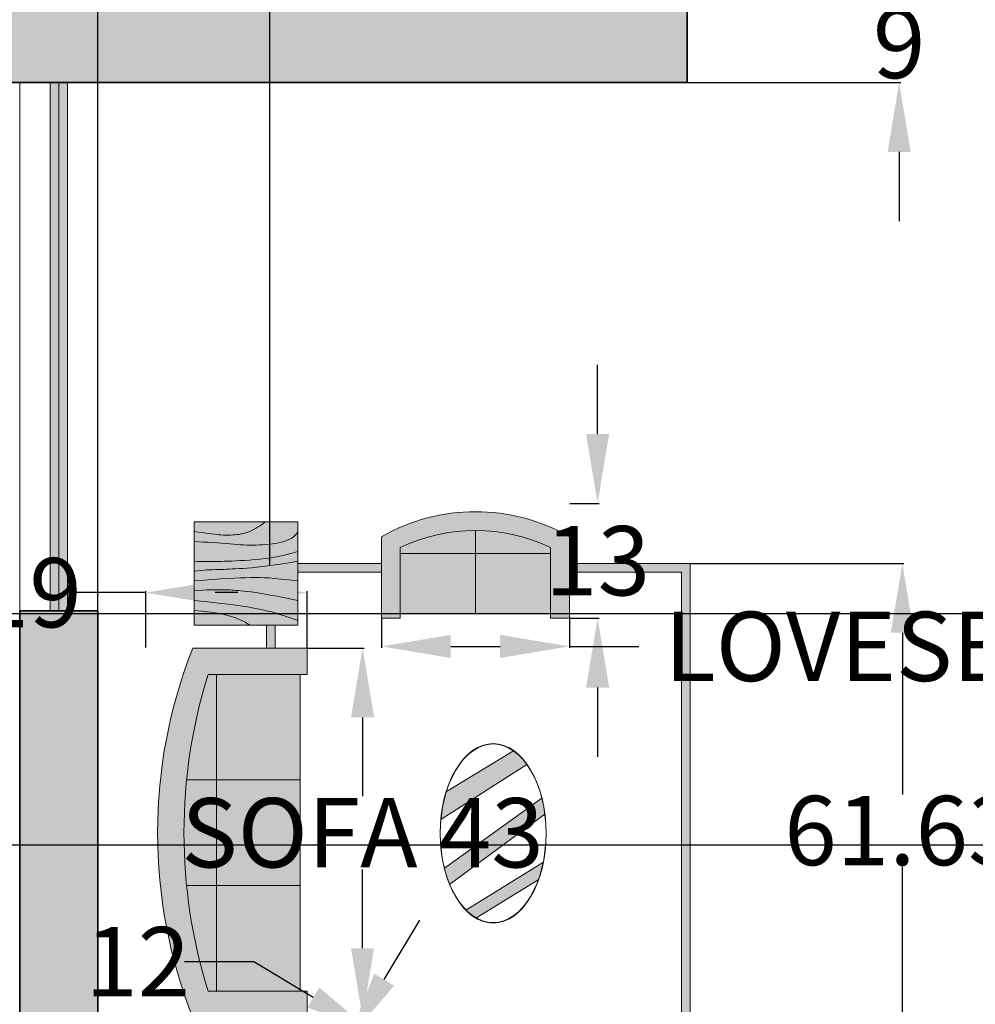
# Model space of a CAD drawing. Units: inches. Extents: x -52 to 678, y 23 to 685.
# Tile 4 of 11: x 189 to 299, y 221 to 334. Entities that reach past the tile are written whole.
import ezdxf

# ---------------------------------------------------------------- set-up
doc = ezdxf.new("R2010")
doc.units = ezdxf.units.IN
doc.header["$MEASUREMENT"] = 0
for name, color, linetype, lineweight in [('A-ANNO-DIMS', 2, 'Continuous', 18), ('A-FURN', 8, 'Continuous', 18), ('A-FURN-PATT', 252, 'Continuous', 13), ('A-GLAZ', 4, 'Continuous', 18), ('A-WALL', 7, 'Continuous', 35)]:
    doc.layers.add(name, color=color, linetype=linetype, lineweight=lineweight)
doc.layers.add('A-GLAZ-PATT', color=18, linetype='Continuous', lineweight=13, true_color=0x000000)
doc.layers.add('A-WALL-PATT', color=18, linetype='Continuous', lineweight=13, true_color=0x000000)
doc.styles.get("Standard").update_dxf_attribs({"font": 'arial.ttf'})
doc.dimstyles.get("Standard").update_dxf_attribs({"dimtxt": 8, "dimasz": 8, "dimexe": 0.18, "dimexo": 0.0625, "dimgap": 0.09, "dimtad": 0, "dimtih": 1, "dimtoh": 1, "dimdec": 0, "dimzin": 0, "dimdsep": 46, "dimlunit": 3, "dimtxsty": 'Standard', "dimcen": 0.09, "dimadec": 0, "dimazin": 0, "dimtfac": 1, "dimtdec": 0, "dimtofl": 0, "dimtmove": 0, "dimatfit": 3, "dimfxl": 1, "dimtolj": 1, "dimtzin": 0, "dimarcsym": 0})

# ---------------------------------------------------------------- blocks, each defined once
blk = doc.blocks.new('Sofa - Roundback Loveseat 5 ft.')
for p, q in [((0, -32.44198), (0, -5.99998)), ((-24, -33.99998), (-24, -11.46958)), ((24.00004, -33.99998), (24.00004, -11.46958)), ((-23.9998, -13.38178), (23.99986, -13.38178)), ((-24, -32.44198), (24.00004, -32.44198))]:
    blk.add_line(p, q)
for points in [[(-24, -33.99998), (-30, -33.99998), (-30, -7.99998)], [(30.00004, -7.99998), (30.00004, -33.99998), (24.00004, -33.99998)]]:
    blk.add_lwpolyline(points)
for centre, radius, start, end in [((0, -60.24998), 60.24998, 60.13715, 119.8628), ((0, -61.38438), 55.38444, 64.32083, 115.6792)]:
    blk.add_arc(centre, radius, start, end)
blk = doc.blocks.new('Sofa - Roundback 7 ft.')
for p, q in [((-12.00002, -32.4421), (-12.00003, -6.5971)), ((11.99997, -32.4421), (11.99998, -6.5971)), ((-36.000027, -34), (-36.000027, -11.4696)), ((-35.999844, -13.3819), (35.9998, -13.3819)), ((35.99998, -34), (35.99998, -11.4696)), ((-36.000027, -32.4421), (35.99998, -32.4421))]:
    blk.add_line(p, q)
for points in [[(-36.000027, -34), (-42.000027, -34), (-42.000027, -8)], [(41.99998, -8), (41.99998, -34), (35.99998, -34)]]:
    blk.add_lwpolyline(points)
for centre, radius, start, end in [((0, -114.25), 114.25, 68.43141, 111.5686), ((-0.00001, -127.1968), 121.1968, 72.72033, 107.2797)]:
    blk.add_arc(centre, radius, start, end)
blk = doc.blocks.new('Table - Square Woodgrain 42 x 42 in.')
blk.add_line((0, -42), (42, -42))
for points in [[(0, -4), (1.704, -4.2172), (3.2358, -4.4188), (4.615, -4.604), (5.8615, -4.7721), (6.9951, -4.9224), (8.0357, -5.0541), (9.0031, -5.1667), (9.9171, -5.2594), (10.7951, -5.3316), (11.6445, -5.3836), (12.4702, -5.4157), (13.277, -5.4283), (14.0698, -5.4217), (14.8535, -5.3964), (15.6331, -5.3526), (16.4133, -5.2908), (17.1986, -5.2103), (17.9913, -5.1062), (18.793, -4.9727), (19.6056, -4.8038), (20.4307, -4.5937), (21.2701, -4.3365), (22.1256, -4.0262), (22.9989, -3.6571), (23.888, -3.2272), (24.7756, -2.7516), (25.6408, -2.2491), (26.4624, -1.7387), (27.2195, -1.2395), (27.891, -0.7703), (28.456, -0.3501), (28.8934, 0.002)], [(0, -42), (0, 0), (42, 0), (42, -42)], [(0, -8), (1.8203, -8.1001), (3.6741, -8.2149), (5.5411, -8.3408), (7.4011, -8.4741), (9.2339, -8.6112), (11.0193, -8.7484), (12.7371, -8.8821), (14.3671, -9.0086), (15.8954, -9.1246), (17.3337, -9.2278), (18.6997, -9.3159), (20.0116, -9.387), (21.2871, -9.4389), (22.5442, -9.4696), (23.8008, -9.477), (25.0749, -9.459), (26.3791, -9.4137), (27.7049, -9.3403), (29.0383, -9.2382), (30.3655, -9.1068), (31.6728, -8.9455), (32.9461, -8.7535), (34.1717, -8.5304), (35.3358, -8.2756), (36.4268, -7.9863), (37.443, -7.6521), (38.3849, -7.2603), (39.253, -6.7986), (40.048, -6.2542), (40.7705, -5.6147), (41.421, -4.8674), (42, -4)], [(42, -12), (39.1784, -12.8621), (36.4519, -13.5654), (33.8246, -14.1294), (31.3004, -14.5731), (28.8832, -14.9161), (26.577, -15.1775), (24.3858, -15.3768), (22.3136, -15.5332), (20.3622, -15.6632), (18.5254, -15.7718), (16.7947, -15.8612), (15.1618, -15.9338), (13.6183, -15.9916), (12.1558, -16.0369), (10.7659, -16.0718), (9.4403, -16.0987), (8.1703, -16.1191), (6.9461, -16.1325), (5.7577, -16.1377), (4.595, -16.1335), (3.4479, -16.1188), (2.3064, -16.0924), (1.1604, -16.0532), (0, -16)], [(42, -16), (37.6529, -16.7365), (33.8802, -17.329), (30.6179, -17.7961), (27.8015, -18.1561), (25.3668, -18.4275), (23.2497, -18.6288), (21.3859, -18.7785), (19.7111, -18.8949), (18.1693, -18.9939), (16.7375, -19.0795), (15.401, -19.1534), (14.1449, -19.217), (12.9544, -19.2717), (11.8148, -19.3191), (10.7113, -19.3606), (9.6291, -19.3976), (8.5534, -19.4323), (7.47, -19.4689), (6.3643, -19.5122), (5.222, -19.5672), (4.0288, -19.6386), (2.7703, -19.7313), (1.4321, -19.8501), (0, -20)], [(0, -24), (3.9243, -23.6805), (7.4766, -23.4138), (10.6891, -23.1954), (13.5943, -23.0205), (16.2247, -22.8847), (18.6125, -22.7832), (20.7903, -22.7116), (22.7903, -22.6651), (24.6563, -22.642), (26.4764, -22.6507), (28.35, -22.7024), (30.3766, -22.8084), (32.6555, -22.98), (35.2861, -23.2283), (38.3678, -23.5645), (42, -24)], [(42, -32), (37.392, -31.017), (33.4585, -30.2231), (30.1291, -29.5949), (27.3334, -29.109), (25.0009, -28.742), (23.0612, -28.4707), (21.4439, -28.2716), (20.0786, -28.1215), (18.8998, -28.0002), (17.8609, -27.9014), (16.9206, -27.8219), (16.0371, -27.7588), (15.1691, -27.709), (14.2748, -27.6693), (13.3128, -27.6368), (12.2415, -27.6083), (11.0295, -27.5824), (9.6867, -27.5643), (8.233, -27.5608), (6.6884, -27.5787), (5.0728, -27.6248), (3.4062, -27.7058), (1.7086, -27.8286), (0, -28)], [(0, -32), (5.4026, -32.5358), (9.9494, -33.019), (13.7424, -33.4553), (16.8834, -33.8505), (19.4743, -34.2106), (21.6171, -34.5413), (23.4136, -34.8486), (24.9657, -35.1382), (26.3614, -35.4156), (27.6332, -35.6841), (28.7995, -35.9467), (29.8788, -36.2064), (30.8897, -36.4661), (31.8507, -36.7288), (32.7802, -36.9973), (33.6968, -37.2747), (34.6175, -37.5635), (35.5531, -37.8651), (36.5128, -38.1805), (37.506, -38.5108), (38.5421, -38.8568), (39.6302, -39.2197), (40.7797, -39.6004), (42, -40)], [(0, -36), (3.0098, -36.2857), (5.5354, -36.5643), (7.6368, -36.8359), (9.374, -37.1009), (10.807, -37.3597), (11.9957, -37.6126), (13.0002, -37.8599), (13.8804, -38.102), (14.6874, -38.3393), (15.4365, -38.5729), (16.1338, -38.8041), (16.7858, -39.0341), (17.3987, -39.264), (17.9787, -39.4952), (18.5322, -39.7288), (19.0655, -39.9662), (19.5832, -40.2081), (20.0842, -40.4544), (20.5657, -40.7046), (21.0249, -40.9581), (21.459, -41.2144), (21.8653, -41.4731), (22.2409, -41.7335), (22.5831, -41.9951)]]:
    blk.add_lwpolyline(points)
blk = doc.blocks.new('*D21')
at = {"layer": 'A-ANNO-DIMS', "color": 0, "lineweight": -2, "transparency": 16777216}
for p, q in [((230.65, 223.62), (234.77, 230.48)), ((228.24, 215.74), (226.38, 216.85)), ((221.23, 204.07), (219.38, 205.18)), ((215.42, 198.23), (211.3, 191.37)), ((211.3, 191.37), (203.3, 191.37))]:
    blk.add_line(p, q, dxfattribs=at)
at = {"layer": 'A-ANNO-DIMS', "color": 0, "transparency": 16777216}
for points in [[(229.51, 224.3), (231.8, 222.93), (226.54, 216.76)], [(214.28, 198.91), (216.56, 197.54), (219.54, 205.09)]]:
    blk.add_solid(points, dxfattribs=at)
at = {"layer": 'Defpoints', "color": 0, "transparency": 16777216}
for p in [(228.29, 215.71), (219.54, 205.09), (221.29, 204.04)]:
    blk.add_point(p, dxfattribs=at)
at = {"layer": 'A-ANNO-DIMS', "color": 0, "transparency": 16777216, "insert": (172.25, 191.37), "char_height": 8, "attachment_point": 5}
blk.add_mtext('\\A1;ROCKER 14', dxfattribs=at)
blk = doc.blocks.new('*D22')
at = {"layer": 'A-ANNO-DIMS', "color": 0, "lineweight": -2, "transparency": 16777216}
for p, q in [((215.62, 225.69), (207.62, 225.69)), ((222.48, 221.57), (215.62, 225.69)), ((228.32, 215.76), (229.43, 217.61)), ((238.88, 209.42), (239.99, 211.27)), ((246.76, 207), (253.62, 202.89))]:
    blk.add_line(p, q, dxfattribs=at)
at = {"layer": 'A-ANNO-DIMS', "color": 0, "transparency": 16777216}
for points in [[(223.17, 222.72), (221.79, 220.43), (229.34, 217.46)], [(247.45, 208.15), (246.07, 205.86), (239.9, 211.12)]]:
    blk.add_solid(points, dxfattribs=at)
at = {"layer": 'Defpoints', "color": 0, "transparency": 16777216}
for p in [(229.34, 217.46), (228.29, 215.71), (238.85, 209.37)]:
    blk.add_point(p, dxfattribs=at)
at = {"layer": 'A-ANNO-DIMS', "color": 0, "transparency": 16777216, "insert": (202.22, 225.69), "char_height": 8, "attachment_point": 5}
blk.add_mtext('\\A1;12', dxfattribs=at)
blk = doc.blocks.new('*D23')
at = {"layer": 'A-ANNO-DIMS', "color": 0, "lineweight": -2, "transparency": 16777216}
for p, q in [((230.34, 265.26), (230.34, 261.89)), ((252.03, 265.26), (252.03, 261.89)), ((238.34, 262.07), (244.03, 262.07)), ((252.03, 262.07), (260.03, 262.07))]:
    blk.add_line(p, q, dxfattribs=at)
at = {"layer": 'A-ANNO-DIMS', "color": 0, "transparency": 16777216}
for points in [[(238.34, 263.4), (238.34, 260.73), (230.34, 262.07)], [(244.03, 263.4), (244.03, 260.73), (252.03, 262.07)]]:
    blk.add_solid(points, dxfattribs=at)
at = {"layer": 'Defpoints', "color": 0, "transparency": 16777216}
for p in [(230.34, 265.32), (252.03, 265.32), (252.03, 262.07)]:
    blk.add_point(p, dxfattribs=at)
at = {"layer": 'A-ANNO-DIMS', "color": 0, "transparency": 16777216, "insert": (296.68, 262.07), "char_height": 8, "attachment_point": 5}
blk.add_mtext('\\A1;LOVESEAT 22', dxfattribs=at)
blk = doc.blocks.new('*D24')
at = {"layer": 'A-ANNO-DIMS', "color": 0, "lineweight": -2, "transparency": 16777216}
for p, q in [((255.28, 286.57), (255.28, 294.57)), ((252.09, 278.57), (255.46, 278.57)), ((252.09, 265.32), (255.46, 265.32)), ((255.28, 257.32), (255.28, 249.32))]:
    blk.add_line(p, q, dxfattribs=at)
at = {"layer": 'A-ANNO-DIMS', "color": 0, "transparency": 16777216}
for points in [[(253.95, 286.57), (256.61, 286.57), (255.28, 278.57)], [(253.95, 257.32), (256.61, 257.32), (255.28, 265.32)]]:
    blk.add_solid(points, dxfattribs=at)
at = {"layer": 'Defpoints', "color": 0, "transparency": 16777216}
for p in [(252.03, 278.57), (255.28, 278.57), (252.03, 265.32)]:
    blk.add_point(p, dxfattribs=at)
at = {"layer": 'A-ANNO-DIMS', "color": 0, "transparency": 16777216, "insert": (255.28, 271.95), "char_height": 8, "attachment_point": 5}
blk.add_mtext('\\A1;13', dxfattribs=at)
blk = doc.blocks.new('*D25')
at = {"layer": 'A-ANNO-DIMS', "color": 0, "lineweight": -2, "transparency": 16777216}
for p, q in [((221.83, 261.88), (228.34, 261.88)), ((228.16, 253.88), (228.16, 244.8)), ((228.16, 227.25), (228.16, 236.33)), ((221.83, 219.25), (228.34, 219.25))]:
    blk.add_line(p, q, dxfattribs=at)
at = {"layer": 'A-ANNO-DIMS', "color": 0, "transparency": 16777216}
for points in [[(226.83, 253.88), (229.49, 253.88), (228.16, 261.88)], [(226.83, 227.25), (229.49, 227.25), (228.16, 219.25)]]:
    blk.add_solid(points, dxfattribs=at)
at = {"layer": 'Defpoints', "color": 0, "transparency": 16777216}
for p in [(221.77, 261.88), (228.16, 261.88), (221.77, 219.25)]:
    blk.add_point(p, dxfattribs=at)
at = {"layer": 'A-ANNO-DIMS', "color": 0, "transparency": 16777216, "insert": (228.16, 240.57), "char_height": 8, "attachment_point": 5}
blk.add_mtext('\\A1;SOFA 43', dxfattribs=at)
blk = doc.blocks.new('*D26')
at = {"layer": 'A-ANNO-DIMS', "color": 0, "lineweight": -2, "transparency": 16777216}
for p, q in [((203.16, 268.27), (195.16, 268.27)), ((203.16, 261.94), (203.16, 268.45)), ((213.77, 268.27), (211.16, 268.27)), ((221.77, 261.94), (221.77, 268.45))]:
    blk.add_line(p, q, dxfattribs=at)
at = {"layer": 'A-ANNO-DIMS', "color": 0, "transparency": 16777216}
for points in [[(211.16, 269.61), (211.16, 266.94), (203.16, 268.27)], [(213.77, 269.61), (213.77, 266.94), (221.77, 268.27)]]:
    blk.add_solid(points, dxfattribs=at)
at = {"layer": 'Defpoints', "color": 0, "transparency": 16777216}
for p in [(203.16, 268.27), (203.16, 261.88), (221.77, 261.88)]:
    blk.add_point(p, dxfattribs=at)
at = {"layer": 'A-ANNO-DIMS', "color": 0, "transparency": 16777216, "insert": (189.71, 268.27), "char_height": 8, "attachment_point": 5}
blk.add_mtext('\\A1;19', dxfattribs=at)
blk = doc.blocks.new('*D39')
at = {"layer": 'A-ANNO-DIMS', "color": 0, "lineweight": -2, "transparency": 16777216}
for p, q in [((91.61, 327.06), (91.61, 28.49)), ((575.61, 53.06), (575.61, 28.49)), ((99.61, 28.67), (324.53, 28.67)), ((567.61, 28.67), (342.68, 28.67))]:
    blk.add_line(p, q, dxfattribs=at)
at = {"layer": 'A-ANNO-DIMS', "color": 0, "transparency": 16777216}
for points in [[(99.61, 30), (99.61, 27.33), (91.61, 28.67)], [(567.61, 30), (567.61, 27.33), (575.61, 28.67)]]:
    blk.add_solid(points, dxfattribs=at)
at = {"layer": 'Defpoints', "color": 0, "transparency": 16777216}
for p in [(91.61, 327.13), (575.61, 53.13), (575.61, 28.67)]:
    blk.add_point(p, dxfattribs=at)
at = {"layer": 'A-ANNO-DIMS', "color": 0, "transparency": 16777216, "insert": (333.61, 28.67), "char_height": 8, "attachment_point": 5}
blk.add_mtext('\\A1;484', dxfattribs=at)
blk = doc.blocks.new('*D59')
at = {"layer": 'A-ANNO-DIMS', "color": 0, "lineweight": -2, "transparency": 16777216}
for p, q in [((290.07, 344.13), (290.07, 352.13)), ((265.67, 336.13), (290.25, 336.13)), ((265.67, 327.13), (290.25, 327.13)), ((290.07, 319.13), (290.07, 311.13))]:
    blk.add_line(p, q, dxfattribs=at)
at = {"layer": 'A-ANNO-DIMS', "color": 0, "transparency": 16777216}
for points in [[(288.73, 344.13), (291.4, 344.13), (290.07, 336.13)], [(288.73, 319.13), (291.4, 319.13), (290.07, 327.13)]]:
    blk.add_solid(points, dxfattribs=at)
at = {"layer": 'Defpoints', "color": 0, "transparency": 16777216}
for p in [(265.61, 336.13), (265.61, 327.13), (290.07, 327.13)]:
    blk.add_point(p, dxfattribs=at)
at = {"layer": 'A-ANNO-DIMS', "color": 0, "transparency": 16777216, "insert": (290.07, 331.63), "char_height": 8, "attachment_point": 5}
blk.add_mtext('\\A1;9', dxfattribs=at)
blk = doc.blocks.new('*D100')
at = {"layer": 'A-ANNO-DIMS', "color": 0, "lineweight": -2, "transparency": 16777216}
for p, q in [((519.99, 265.81), (66.97, 265.81)), ((67.15, 257.81), (67.15, 256.65)), ((67.15, 247.13), (67.15, 248.3)), ((521.98, 239.13), (66.97, 239.13))]:
    blk.add_line(p, q, dxfattribs=at)
at = {"layer": 'A-ANNO-DIMS', "color": 0, "transparency": 16777216}
for points in [[(65.81, 257.81), (68.48, 257.81), (67.15, 265.81)], [(65.81, 247.13), (68.48, 247.13), (67.15, 239.13)]]:
    blk.add_solid(points, dxfattribs=at)
at = {"layer": 'Defpoints', "color": 0, "transparency": 16777216}
for p in [(520.05, 265.81), (67.15, 239.13), (522.04, 239.13)]:
    blk.add_point(p, dxfattribs=at)
at = {"layer": 'A-ANNO-DIMS', "color": 0, "transparency": 16777216, "insert": (67.15, 252.47), "char_height": 8, "attachment_point": 5}
blk.add_mtext('\\A1;26.69', dxfattribs=at)
blk = doc.blocks.new('*D102')
at = {"layer": 'A-ANNO-DIMS', "color": 0, "lineweight": -2, "transparency": 16777216}
for p, q in [((266.04, 271.64), (290.62, 271.64)), ((290.44, 263.64), (290.44, 245)), ((290.44, 218.01), (290.44, 236.65)), ((266.04, 210.01), (290.62, 210.01))]:
    blk.add_line(p, q, dxfattribs=at)
at = {"layer": 'A-ANNO-DIMS', "color": 0, "transparency": 16777216}
for points in [[(289.1, 263.64), (291.77, 263.64), (290.44, 271.64)], [(289.1, 218.01), (291.77, 218.01), (290.44, 210.01)]]:
    blk.add_solid(points, dxfattribs=at)
at = {"layer": 'Defpoints', "color": 0, "transparency": 16777216}
for p in [(265.98, 271.64), (265.98, 210.01), (290.44, 210.01)]:
    blk.add_point(p, dxfattribs=at)
at = {"layer": 'A-ANNO-DIMS', "color": 0, "transparency": 16777216, "insert": (290.44, 240.82), "char_height": 8, "attachment_point": 5}
blk.add_mtext('\\A1;61.63', dxfattribs=at)
blk = doc.blocks.new('*D103')
at = {"layer": 'A-ANNO-DIMS', "color": 0, "lineweight": -2, "transparency": 16777216}
for p, q in [((197.61, 266.24), (197.61, 549.77)), ((205.61, 549.59), (209.46, 549.59)), ((217.46, 271.45), (217.46, 549.77)), ((217.46, 549.59), (225.46, 549.59))]:
    blk.add_line(p, q, dxfattribs=at)
at = {"layer": 'A-ANNO-DIMS', "color": 0, "transparency": 16777216}
for points in [[(205.61, 550.92), (205.61, 548.25), (197.61, 549.59)], [(209.46, 550.92), (209.46, 548.25), (217.46, 549.59)]]:
    blk.add_solid(points, dxfattribs=at)
at = {"layer": 'Defpoints', "color": 0, "transparency": 16777216}
for p in [(217.46, 549.59), (217.46, 271.39), (197.61, 266.17)]:
    blk.add_point(p, dxfattribs=at)
at = {"layer": 'A-ANNO-DIMS', "color": 0, "transparency": 16777216, "insert": (241.78, 549.59), "char_height": 8, "attachment_point": 5}
blk.add_mtext('\\A1;19.856', dxfattribs=at)

msp = doc.modelspace()

# ---------------------------------------------------------------- hatches: boundary and pattern name
at = {"layer": 'A-FURN-PATT'}
h = msp.add_hatch(color=256, dxfattribs=at)
h.dxf.hatch_style = 1
h.paths.add_polyline_path([(230.3425, 265.3206), (232.5109, 265.3206), (232.5109, 273.4629, -0.22792319), (249.8583, 273.4629), (249.8583, 265.3206), (252.0267, 265.3206), (252.0267, 274.717, 0.26666697), (230.3425, 274.7171)])
h = msp.add_hatch(color=256, dxfattribs=at)
h.dxf.hatch_style = 1
h.paths.add_polyline_path([(212.7536, 274.908), (212.9766, 274.9152), (213.1983, 274.9276), (213.4203, 274.9452), (213.6437, 274.9681), (213.8692, 274.9977), (214.0972, 275.0357), (214.3284, 275.0837), (214.5631, 275.1435), (214.8018, 275.2166), (215.0452, 275.3049), (215.2936, 275.4099), (215.5465, 275.5322), (215.799, 275.6675), (216.0451, 275.8104), (216.2788, 275.9556), (216.4942, 276.0976), (216.6852, 276.2311), (216.8459, 276.3506), (216.9696, 276.4502), (208.7514, 276.4502), (208.7514, 275.3124), (209.2361, 275.2506), (209.6718, 275.1932), (210.0641, 275.1406), (210.4187, 275.0927), (210.7412, 275.05), (211.0372, 275.0125), (211.3124, 274.9805), (211.5724, 274.9541), (211.8221, 274.9336), (212.0638, 274.9188), (212.2986, 274.9097), (212.5281, 274.9061)])
h = msp.add_hatch(color=256, dxfattribs=at)
h.dxf.hatch_style = 1
h.paths.add_polyline_path([(219.1133, 274.1784), (219.4024, 274.2735), (219.6703, 274.3849), (219.9172, 274.5163), (220.1434, 274.6711), (220.3489, 274.8531), (220.5339, 275.0656), (220.6986, 275.3124), (220.6986, 276.4502), (216.9696, 276.4502), (216.8459, 276.3506), (216.6852, 276.2311), (216.4942, 276.0976), (216.2788, 275.9556), (216.0451, 275.8104), (215.799, 275.6675), (215.5465, 275.5322), (215.2936, 275.4099), (215.0452, 275.3049), (214.8018, 275.2166), (214.5631, 275.1435), (214.3284, 275.0837), (214.0972, 275.0357), (213.8692, 274.9977), (213.6437, 274.9681), (213.4203, 274.9452), (213.1983, 274.9276), (212.9766, 274.9152), (212.7536, 274.908), (212.5281, 274.9061), (212.2986, 274.9097), (212.0638, 274.9188), (211.8221, 274.9336), (211.5724, 274.9541), (211.3124, 274.9805), (211.0372, 275.0125), (210.7412, 275.05), (210.4187, 275.0927), (210.0641, 275.1406), (209.6718, 275.1932), (209.2361, 275.2506), (208.7514, 275.3124), (208.7514, 274.1745), (209.2692, 274.1461), (209.7965, 274.1134), (210.3276, 274.0776), (210.8567, 274.0397), (211.378, 274.0007), (211.8859, 273.9616), (212.3746, 273.9236), (212.8382, 273.8876), (213.273, 273.8546), (213.6821, 273.8253), (214.0707, 273.8002), (214.4438, 273.78), (214.8067, 273.7652), (215.1643, 273.7565), (215.5217, 273.7544), (215.8841, 273.7595), (216.2551, 273.7724), (216.6323, 273.7933), (217.0116, 273.8223), (217.3891, 273.8597), (217.761, 273.9056), (218.1232, 273.9602), (218.4718, 274.0237), (218.803, 274.0961)])
h = msp.add_hatch(color=256, dxfattribs=at)
h.dxf.hatch_style = 1
h.paths.add_polyline_path([(212.6252, 271.9013), (213.0643, 271.9177), (213.5288, 271.9383), (214.0211, 271.9638), (214.5436, 271.9947), (215.0987, 272.0316), (215.6881, 272.0761), (216.3114, 272.1328), (216.9675, 272.2072), (217.655, 272.3048), (218.3731, 272.431), (219.1204, 272.5914), (219.896, 272.7915), (220.6986, 273.0367), (220.6986, 275.3124), (220.5339, 275.0656), (220.3489, 274.8531), (220.1434, 274.6711), (219.9172, 274.5163), (219.6703, 274.3849), (219.4024, 274.2735), (219.1133, 274.1784), (218.803, 274.0961), (218.4718, 274.0237), (218.1232, 273.9602), (217.761, 273.9056), (217.3891, 273.8597), (217.0116, 273.8223), (216.6323, 273.7933), (216.2551, 273.7724), (215.8841, 273.7595), (215.5217, 273.7544), (215.1643, 273.7565), (214.8067, 273.7652), (214.4438, 273.78), (214.0707, 273.8002), (213.6821, 273.8253), (213.273, 273.8546), (212.8382, 273.8876), (212.3746, 273.9236), (211.8859, 273.9616), (211.378, 274.0007), (210.8567, 274.0397), (210.3276, 274.0776), (209.7965, 274.1134), (209.2692, 274.1461), (208.7514, 274.1745), (208.7514, 271.8989), (209.0815, 271.8837), (209.4074, 271.8726), (209.7322, 271.8651), (210.0585, 271.8609), (210.3892, 271.8597), (210.7272, 271.8612), (211.0755, 271.865), (211.4367, 271.8708), (211.8138, 271.8784), (212.2092, 271.8884)])
h = msp.add_hatch(color=256, dxfattribs=at)
h.dxf.hatch_style = 1
h.paths.add_polyline_path([(241.1846, 272.7721), (241.1846, 275.4399, 0.11251869), (232.5109, 273.4629), (232.5109, 272.7721)])
h = msp.add_hatch(color=256, dxfattribs=at)
h.dxf.hatch_style = 1
h.paths.add_polyline_path([(249.8583, 272.7721), (249.8583, 273.4629, 0.11251889), (241.1846, 275.4399), (241.1846, 272.7721)])
h = msp.add_hatch(color=256, dxfattribs=at)
h.dxf.hatch_style = 1
h.paths.add_polyline_path([(218.3889, 271.5208), (219.4621, 271.6894), (220.6986, 271.8989), (220.6986, 273.0367), (219.896, 272.7915), (219.1204, 272.5914), (218.3731, 272.431), (217.655, 272.3048), (216.9675, 272.2072), (216.3114, 272.1328), (215.6881, 272.0761), (215.0987, 272.0316), (214.5436, 271.9947), (214.0211, 271.9638), (213.5288, 271.9383), (213.0643, 271.9177), (212.6252, 271.9013), (212.2092, 271.8884), (211.8138, 271.8784), (211.4367, 271.8708), (211.0755, 271.865), (210.7272, 271.8612), (210.3892, 271.8597), (210.0585, 271.8609), (209.7322, 271.8651), (209.4074, 271.8726), (209.0815, 271.8837), (208.7514, 271.8989), (208.7514, 270.761), (209.1587, 270.8037), (209.5394, 270.8375), (209.8974, 270.8638), (210.2368, 270.8841), (210.5618, 270.8998), (210.8763, 270.9121), (211.1845, 270.9225), (211.4905, 270.9324), (211.7983, 270.9429), (212.1122, 270.9547), (212.4364, 270.9682), (212.775, 270.9838), (213.1323, 271.0019), (213.5125, 271.0229), (213.9198, 271.0472), (214.3584, 271.0754), (214.8348, 271.1085), (215.365, 271.1511), (215.9672, 271.2083), (216.6598, 271.2855), (217.4609, 271.3879)])
h = msp.add_hatch(color=256, dxfattribs=at)
h.dxf.hatch_style = 1
h.paths.add_polyline_path([(241.1846, 265.8836), (241.1846, 272.7721), (232.5109, 272.7721), (232.5109, 265.8836)])
h = msp.add_hatch(color=256, dxfattribs=at)
h.dxf.hatch_style = 1
h.paths.add_polyline_path([(249.8583, 265.8836), (249.8583, 272.7721), (241.1846, 272.7721), (241.1846, 265.8836)])
h = msp.add_hatch(color=256, dxfattribs=at)
h.dxf.hatch_style = 1
h.paths.add_polyline_path([(212.4364, 270.9682), (212.1122, 270.9547), (211.7983, 270.9429), (211.4905, 270.9324), (211.1845, 270.9225), (210.8763, 270.9121), (210.5618, 270.8998), (210.2368, 270.8841), (209.8974, 270.8638), (209.5394, 270.8375), (209.1587, 270.8037), (208.7514, 270.761), (208.7514, 269.6232), (209.8677, 269.7141), (210.8782, 269.7899), (211.792, 269.8521), (212.6184, 269.9018), (213.3666, 269.9404), (214.0459, 269.9693), (214.6654, 269.9897), (215.2343, 270.0029), (215.7651, 270.0095), (216.2828, 270.007), (216.8158, 269.9923), (217.3923, 269.9622), (218.0405, 269.9133), (218.7888, 269.8427), (219.6654, 269.7471), (220.6986, 269.6232), (220.6986, 271.8989), (219.4621, 271.6894), (218.3889, 271.5208), (217.4609, 271.3879), (216.6598, 271.2855), (215.9672, 271.2083), (215.365, 271.1511), (214.8348, 271.1085), (214.3584, 271.0754), (213.9198, 271.0472), (213.5125, 271.0229), (213.1323, 271.0019), (212.775, 270.9838)])
h = msp.add_hatch(color=256, dxfattribs=at)
h.dxf.hatch_style = 1
h.paths.add_polyline_path([(230.3425, 270.638), (230.3425, 271.638), (220.6986, 271.638), (220.6986, 270.638)])
h = msp.add_hatch(color=256, dxfattribs=at)
h.dxf.hatch_style = 1
h.paths.add_polyline_path([(264.9763, 211.0118), (232.1935, 211.0118), (232.532, 210.8087), (233.7567, 210.0739), (236.7223, 210.0739), (237.0272, 210.4629), (237.6755, 210.0739), (265.9763, 210.0118), (265.9763, 211.0118), (265.9763, 271.638), (264.9763, 271.638), (252.0267, 271.638), (252.0267, 270.638), (264.9763, 270.638)])
h = msp.add_hatch(color=256, dxfattribs=at)
h.dxf.hatch_style = 1
h.paths.add_polyline_path([(217.3923, 269.9622), (216.8158, 269.9923), (216.2828, 270.007), (215.7651, 270.0095), (215.2343, 270.0029), (214.6654, 269.9897), (214.0459, 269.9693), (213.3666, 269.9404), (212.6184, 269.9018), (211.792, 269.8521), (210.8782, 269.7899), (209.8677, 269.7141), (208.7514, 269.6232), (208.7514, 268.4854), (209.2374, 268.5341), (209.7203, 268.569), (210.1944, 268.5921), (210.6539, 268.6052), (211.0933, 268.6103), (211.5068, 268.6093), (211.8888, 268.6041), (212.2336, 268.5968), (212.5383, 268.5887), (212.812, 268.5794), (213.0664, 268.5681), (213.3133, 268.554), (213.5646, 268.536), (213.8321, 268.5134), (214.1276, 268.4853), (214.4629, 268.4508), (214.8513, 268.4081), (215.3113, 268.3515), (215.8631, 268.2743), (216.5266, 268.1699), (217.3219, 268.0317), (218.2689, 267.853), (219.3879, 267.6271), (220.6986, 267.3475), (220.6986, 269.6232), (219.6654, 269.7471), (218.7888, 269.8427), (218.0405, 269.9133)])
h = msp.add_hatch(color=256, dxfattribs=at)
h.dxf.hatch_style = 1
h.paths.add_polyline_path([(212.5383, 268.5887), (212.2336, 268.5968), (211.8888, 268.6041), (211.5068, 268.6093), (211.0933, 268.6103), (210.6539, 268.6052), (210.1944, 268.5921), (209.7203, 268.569), (209.2374, 268.5341), (208.7514, 268.4854), (208.7514, 267.3475), (210.2882, 267.1951), (211.5816, 267.0577), (212.6605, 266.9335), (213.554, 266.8211), (214.291, 266.7187), (214.9005, 266.6246), (215.4116, 266.5372), (215.8531, 266.4548), (216.2501, 266.3759), (216.6119, 266.2995), (216.9436, 266.2248), (217.2507, 266.151), (217.5382, 266.0771), (217.8116, 266.0024), (218.076, 265.926), (218.3367, 265.8471), (218.5986, 265.7649), (218.8648, 265.6791), (219.1378, 265.5894), (219.4203, 265.4955), (219.715, 265.397), (220.0245, 265.2938), (220.3515, 265.1855), (220.6986, 265.0719), (220.6986, 267.3475), (219.3879, 267.6271), (218.2689, 267.853), (217.3219, 268.0317), (216.5266, 268.1699), (215.8631, 268.2743), (215.3113, 268.3515), (214.8513, 268.4081), (214.4629, 268.4508), (214.1276, 268.4853), (213.8321, 268.5134), (213.5646, 268.536), (213.3133, 268.554), (213.0664, 268.5681), (212.812, 268.5794)])
h = msp.add_hatch(color=256, dxfattribs=at)
h.dxf.hatch_style = 1
h.paths.add_polyline_path([(215.8531, 266.4548), (215.4116, 266.5372), (214.9005, 266.6246), (214.291, 266.7187), (213.554, 266.8211), (212.6605, 266.9335), (211.5816, 267.0577), (210.2882, 267.1951), (208.7514, 267.3475), (208.7514, 266.2097), (209.6075, 266.1284), (210.326, 266.0492), (210.9237, 265.9719), (211.4179, 265.8965), (211.8255, 265.8229), (212.1637, 265.751), (212.4494, 265.6806), (212.6998, 265.6118), (212.9293, 265.5443), (213.1424, 265.4778), (213.3408, 265.412), (213.5262, 265.3466), (213.7006, 265.2812), (213.8656, 265.2154), (214.023, 265.149), (214.1747, 265.0815), (214.322, 265.0127), (214.4645, 264.9426), (214.6015, 264.8714), (214.7321, 264.7993), (214.8556, 264.7264), (214.9711, 264.6528), (215.078, 264.5787), (215.1772, 264.5029), (220.6986, 264.5029), (220.6986, 265.0719), (220.3515, 265.1855), (220.0245, 265.2938), (219.715, 265.397), (219.4203, 265.4955), (219.1378, 265.5894), (218.8648, 265.6791), (218.5986, 265.7649), (218.3367, 265.8471), (218.076, 265.926), (217.8116, 266.0024), (217.5382, 266.0771), (217.2507, 266.151), (216.9436, 266.2248), (216.6119, 266.2995), (216.2501, 266.3759)])
h = msp.add_hatch(color=256, dxfattribs=at)
h.dxf.hatch_style = 1
h.paths.add_polyline_path([(211.4179, 265.8965), (210.9237, 265.9719), (210.326, 266.0492), (209.6075, 266.1284), (208.7514, 266.2097), (208.7514, 264.5029), (215.1772, 264.5029), (215.078, 264.5787), (214.9711, 264.6528), (214.8556, 264.7264), (214.7321, 264.7993), (214.6015, 264.8714), (214.4645, 264.9426), (214.322, 265.0127), (214.1747, 265.0815), (214.023, 265.149), (213.8656, 265.2154), (213.7006, 265.2812), (213.5262, 265.3466), (213.3408, 265.412), (213.1424, 265.4778), (212.9293, 265.5443), (212.6998, 265.6118), (212.4494, 265.6806), (212.1637, 265.751), (211.8255, 265.8229)])
h = msp.add_hatch(color=256, dxfattribs=at)
h.dxf.hatch_style = 1
h.paths.add_polyline_path([(218.0681, 264.5029), (217.0681, 264.5029), (217.0681, 261.8802), (218.0681, 261.8802)])
h = msp.add_hatch(color=256, dxfattribs=at)
h.dxf.hatch_style = 1
h.paths.add_polyline_path([(221.7669, 219.2523), (221.7669, 222.2971), (210.3335, 222.2971, -0.15194781), (210.3335, 258.8353), (221.7669, 258.8353), (221.7669, 261.8802), (208.5725, 261.8802, 0.19047621), (208.5725, 219.2523)])
h = msp.add_hatch(color=256, dxfattribs=at)
h.dxf.hatch_style = 1
h.paths.add_polyline_path([(211.3037, 258.8353), (210.3335, 258.8353, 0.05064665), (207.8598, 246.6559), (211.3037, 246.6559)])
h = msp.add_hatch(color=256, dxfattribs=at)
h.dxf.hatch_style = 1
h.paths.add_polyline_path([(220.9763, 258.8353), (211.3037, 258.8353), (211.3037, 246.6559), (220.9763, 246.6559)])
h = msp.add_hatch(color=256, dxfattribs=at)
h.dxf.hatch_style = 1
edge = h.paths.add_edge_path()
edge.add_ellipse((243.2355, 240.4812), major_axis=(0, -10.3299), ratio=0.59139781, start_angle=153.9031, end_angle=166.335936)
edge.add_line((245.5582, 250.0354), (237.8417, 245.3316))
edge.add_ellipse((243.2355, 240.4812), major_axis=(0, -10.3299), ratio=0.59139781, start_angle=228.036298, end_angle=254.882425)
edge.add_line((237.2029, 242.1109), (247.1323, 248.4367))
h = msp.add_hatch(color=256, dxfattribs=at)
h.dxf.hatch_style = 1
h.paths.add_polyline_path([(207.8598, 234.4765), (211.3037, 234.4765), (211.3037, 246.6559), (207.8598, 246.6559, 0.04962821)])
h = msp.add_hatch(color=256, dxfattribs=at)
h.dxf.hatch_style = 1
h.paths.add_polyline_path([(211.3037, 246.6559), (211.3037, 234.4765), (220.9763, 234.4765), (220.9763, 246.6559)])
h = msp.add_hatch(color=256, dxfattribs=at)
h.dxf.hatch_style = 1
edge = h.paths.add_edge_path()
edge.add_ellipse((243.2355, 240.4812), major_axis=(0, -10.3299), ratio=0.59139781, start_angle=110.661741, end_angle=126.015557)
edge.add_line((248.8479, 244.5612), (237.599, 236.497))
edge.add_ellipse((243.2355, 240.4812), major_axis=(0, -10.3299), ratio=0.59139781, start_angle=305.254682, end_angle=319.39785)
edge.add_line((238.2071, 234.6149), (249.1981, 242.7297))
h = msp.add_hatch(color=256, dxfattribs=at)
h.dxf.hatch_style = 1
edge = h.paths.add_edge_path()
edge.add_ellipse((243.2355, 240.4812), major_axis=(0, -10.3299), ratio=0.59139781, start_angle=44.785009, end_angle=60.389568)
edge.add_line((249.0262, 237.1902), (240.0714, 231.6447))
edge.add_ellipse((243.2355, 240.4812), major_axis=(0, -10.3299), ratio=0.59139781, start_angle=340.29905, end_angle=348.403739)
edge.add_line((241.2329, 230.722), (248.4836, 235.1935))
h = msp.add_hatch(color=256, dxfattribs=at)
h.dxf.hatch_style = 1
h.paths.add_polyline_path([(211.3037, 234.4765), (207.8598, 234.4765, 0.05064665), (210.3335, 222.2971), (211.3037, 222.2971)])
h = msp.add_hatch(color=256, dxfattribs=at)
h.dxf.hatch_style = 1
h.paths.add_polyline_path([(220.9763, 234.4765), (211.3037, 234.4765), (211.3037, 222.2971), (220.9763, 222.2971)])
at = {"layer": 'A-GLAZ-PATT'}
h = msp.add_hatch(color=256, dxfattribs=at)
h.dxf.hatch_style = 1
h.paths.add_polyline_path([(193.1053, 327.1267), (192.1053, 327.1267), (192.1053, 266.1726), (193.1053, 266.1726)])
h = msp.add_hatch(color=256, dxfattribs=at)
h.dxf.hatch_style = 1
h.paths.add_polyline_path([(194.1053, 327.1267), (193.1053, 327.1267), (193.1053, 266.1726), (194.1053, 266.1726)])
at = {"layer": 'A-WALL-PATT'}
h = msp.add_hatch(color=256, dxfattribs=at)
h.dxf.hatch_style = 1
h.paths.add_polyline_path([(265.6053, 327.1267), (265.6053, 336.1267), (170.301, 336.1267), (170.301, 327.1267)])
h = msp.add_hatch(color=256, dxfattribs=at)
h.dxf.hatch_style = 1
h.paths.add_polyline_path([(188.6053, 212.2126), (197.6053, 212.2126), (197.6053, 266.1726), (188.6053, 266.1726)])

# ---------------------------------------------------------------- linework, layer by layer
at = {"layer": 'A-FURN'}
for p, q in [((220.6986, 271.638), (230.3425, 271.638)), ((252.0267, 271.638), (265.9763, 271.638)), ((265.9763, 271.638), (264.9763, 271.638)), ((265.9763, 271.638), (265.9763, 210.0118)), ((265.9763, 271.638), (265.9763, 270.638)), ((230.3425, 270.638), (220.6986, 270.638)), ((264.9763, 270.638), (252.0267, 270.638)), ((264.9763, 270.638), (264.9763, 211.0118)), ((217.0681, 261.8802), (217.0681, 264.5029)), ((218.0681, 264.5029), (218.0681, 261.8802)), ((245.5582, 250.0354), (237.8417, 245.3316)), ((237.2029, 242.1109), (247.1323, 248.4367)), ((248.8479, 244.5612), (237.599, 236.497)), ((238.2071, 234.6149), (249.1981, 242.7297)), ((249.0262, 237.1902), (240.0714, 231.6447)), ((241.2329, 230.722), (248.4836, 235.1935))]:
    msp.add_line(p, q, dxfattribs=at)
for centre in [(243.2235, 240.5291), (243.2355, 240.4812)]:
    msp.add_ellipse(centre, major_axis=(0, -10.3299), ratio=0.59139781, dxfattribs=at)
at = {"layer": 'A-GLAZ'}
for p, q in [((188.6053, 266.1726), (188.6053, 327.1267)), ((192.1053, 266.1726), (192.1053, 327.1267)), ((193.1053, 266.1726), (193.1053, 327.1267)), ((194.1053, 266.1726), (194.1053, 327.1267)), ((197.6053, 266.1726), (197.6053, 327.1267))]:
    msp.add_line(p, q, dxfattribs=at)
at = {"layer": 'A-WALL'}
for p, q in [((265.6053, 336.1267), (265.6053, 327.1267)), ((170.301, 327.1267), (265.6053, 327.1267)), ((188.6053, 266.1726), (197.6053, 266.1726)), ((188.6053, 212.2126), (188.6053, 266.1726)), ((197.6053, 212.2126), (197.6053, 266.1726))]:
    msp.add_line(p, q, dxfattribs=at)

# ---------------------------------------------------------------- block references
at = {"layer": 'A-FURN'}
for name, p, xscale, yscale, zscale in [('Sofa - Roundback Loveseat 5 ft.', (241.1846, 277.6083), 0.3614033099523193, 0.3614033099523193, 0.3614033099523193), ('Table - Square Woodgrain 42 x 42 in.', (208.7514, 276.4502), 0.2844588312427021, 0.2844588312427021, 0.2844588312427021)]:
    msp.add_blockref(name, p, dxfattribs=dict(at, xscale=xscale, yscale=yscale, zscale=zscale))
at = {"layer": 'A-FURN', "xscale": 0.5074751266368834, "yscale": 0.5074751266368834, "zscale": 0.5074751266368834, "rotation": 90}
msp.add_blockref('Sofa - Roundback 7 ft.', (204.5127, 240.5662), dxfattribs=at)

# ---------------------------------------------------------------- dimensions: what is measured, and where the dimension line sits
at = {"layer": 'A-ANNO-DIMS'}
for base, p1, p2, override, picture, middle in [((217.4609, 549.5867), (197.6053, 266.1726), (217.4609, 271.3879), {"dimdec": 3, "dimlfac": 1, "dimrnd": 0, "dimzin": 0, "dimdsep": 46, "dimlunit": 2}, '*D103', (241.7774, 549.5867)), ((575.6053, 28.6667), (91.6053, 327.1267), (575.6053, 53.1267), {"dimdec": 0, "dimlfac": 1, "dimrnd": 0, "dimzin": 0, "dimdsep": 46, "dimlunit": 2}, '*D39', (333.6053, 28.6667))]:
    dim = msp.add_linear_dim(base=base, p1=p1, p2=p2, dimstyle='Standard', override=override, dxfattribs=at)
    dim.commit()
    dim.dimension.update_dxf_attribs({"geometry": picture, "text_midpoint": middle})
for base, p1, p2, angle, override, picture, middle in [((290.0653, 327.1267), (265.6053, 336.1267), (265.6053, 327.1267), 270, {"dimdec": 0, "dimlfac": 1, "dimrnd": 0, "dimzin": 0, "dimdsep": 46, "dimlunit": 2}, '*D59', (290.0653, 331.6267)), ((255.2793, 278.572), (252.0267, 265.3206), (252.0267, 278.572), 90, {"dimdec": 0, "dimlfac": 1, "dimrnd": 0, "dimzin": 0, "dimdsep": 46, "dimlunit": 2}, '*D24', (255.2793, 271.9463)), ((203.1594, 268.2744), (221.7669, 261.8802), (203.1594, 261.8802), 180, {"dimdec": 0, "dimlfac": 1, "dimrnd": 0, "dimzin": 0, "dimdsep": 46, "dimlunit": 2}, '*D26', (189.7079, 268.2744)), ((290.4363, 210.0118), (265.9763, 271.638), (265.9763, 210.0118), 270, {"dimdec": 2, "dimlfac": 1, "dimrnd": 0, "dimzin": 0, "dimdsep": 46, "dimlunit": 2}, '*D102', (290.4363, 240.8249)), ((67.1453, 239.1267), (520.0511, 265.8145), (522.0448, 239.1267), 90, {"dimdec": 2, "dimlfac": 1, "dimrnd": 0, "dimzin": 0, "dimdsep": 46, "dimlunit": 2}, '*D100', (67.1453, 252.4706)), ((229.339, 217.4565), (238.8501, 209.3691), (228.2887, 215.706), 149.036213, {"dimdec": 0, "dimlfac": 1, "dimrnd": 0, "dimzin": 0, "dimdsep": 46, "dimlunit": 2}, '*D22', (202.2167, 225.6884))]:
    dim = msp.add_linear_dim(base=base, p1=p1, p2=p2, angle=angle, dimstyle='Standard', override=override, dxfattribs=at)
    dim.commit()
    dim.dimension.update_dxf_attribs({"geometry": picture, "text_midpoint": middle})
dim = msp.add_linear_dim(base=(252.0267, 262.0679), p1=(230.3425, 265.3206), p2=(252.0267, 265.3206), text='LOVESEAT <>', dimstyle='Standard', override={"dimdec": 0, "dimlfac": 1, "dimrnd": 0, "dimzin": 0, "dimdsep": 46, "dimlunit": 2}, dxfattribs=at)
dim.commit()
dim.dimension.update_dxf_attribs({"geometry": '*D23', "text_midpoint": (296.6842, 262.0679)})
for base, p1, p2, angle, text, picture, middle in [((228.1611, 261.8802), (221.7669, 219.2523), (221.7669, 261.8802), 90, 'SOFA <>', '*D25', (228.1611, 240.5662)), ((219.5361, 205.0862), (228.2887, 215.706), (221.2866, 204.0359), 239.036213, 'ROCKER <>', '*D21', (172.2483, 191.3664))]:
    dim = msp.add_linear_dim(base=base, p1=p1, p2=p2, angle=angle, text=text, dimstyle='Standard', override={"dimdec": 0, "dimlfac": 1, "dimrnd": 0, "dimzin": 0, "dimdsep": 46, "dimlunit": 2}, dxfattribs=at)
    dim.commit()
    dim.dimension.update_dxf_attribs({"geometry": picture, "text_midpoint": middle})

doc.saveas('drawing.dxf')
